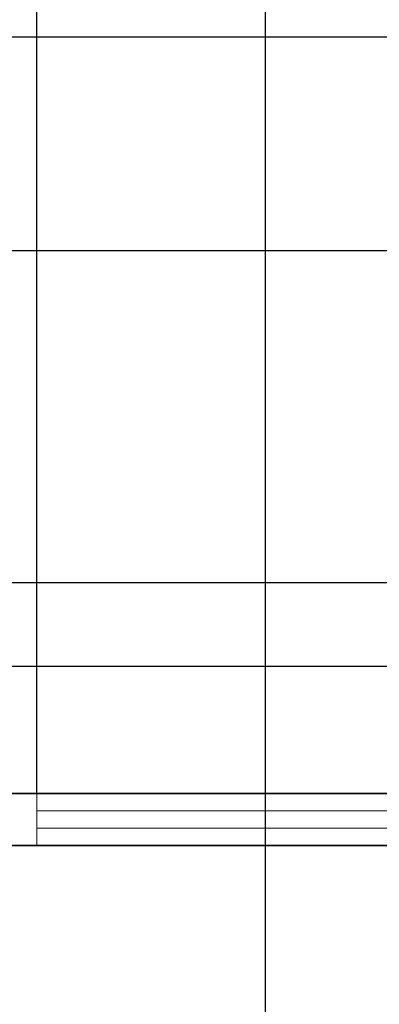
# Model space of a CAD drawing. Units: inches. Extents: x -26 to 385, y 12 to 697.
# Tile 4 of 13: x 192 to 223, y 130 to 215. Entities that reach past the tile are written whole.
import ezdxf

# ---------------------------------------------------------------- set-up
doc = ezdxf.new("R2010")
doc.units = ezdxf.units.IN
doc.header["$MEASUREMENT"] = 0
for name, color, linetype, lineweight in [('A-ANNO-DIMS', 4, 'Continuous', 18), ('A-GLAZ', 5, 'Continuous', 18), ('A-WALL', 40, 'Continuous', 35)]:
    doc.layers.add(name, color=color, linetype=linetype, lineweight=lineweight)
doc.styles.get("Standard").update_dxf_attribs({"font": 'italic8.shx'})
doc.dimstyles.get("Standard").update_dxf_attribs({"dimtxt": 8, "dimasz": 0.18, "dimexe": 0.18, "dimexo": 0.0625, "dimgap": 0.09, "dimtad": 0, "dimtih": 1, "dimtoh": 1, "dimdec": 4, "dimzin": 0, "dimdsep": 46, "dimlunit": 3, "dimtxsty": 'Standard', "dimcen": 0.09, "dimclrd": 2, "dimclre": 3, "dimclrt": 6, "dimadec": 0, "dimazin": 0, "dimtfac": 1, "dimtdec": 4, "dimtofl": 0, "dimtmove": 0, "dimatfit": 3, "dimfxl": 1, "dimtolj": 1, "dimtzin": 0, "dimarcsym": 0})

# ---------------------------------------------------------------- blocks, each defined once
blk = doc.blocks.new('*D28')
at = {"layer": 'A-ANNO-DIMS', "color": 3, "lineweight": -2, "transparency": 16777216}
for p, q in [((141.692, 194.903), (355.559, 194.903)), ((141.692, 158.903), (355.559, 158.903))]:
    blk.add_line(p, q, dxfattribs=at)
at = {"layer": 'A-ANNO-DIMS', "color": 2, "lineweight": -2, "transparency": 16777216}
for p, q in [((355.379, 194.723), (355.379, 181.755)), ((355.379, 159.083), (355.379, 172.052))]:
    blk.add_line(p, q, dxfattribs=at)
at = {"layer": 'A-ANNO-DIMS', "color": 2, "transparency": 16777216}
for points in [[(355.349, 194.723), (355.409, 194.723), (355.379, 194.903)], [(355.349, 159.083), (355.409, 159.083), (355.379, 158.903)]]:
    blk.add_solid(points, dxfattribs=at)
at = {"layer": 'Defpoints', "color": 0, "transparency": 16777216}
for p in [(141.629, 194.903), (355.379, 194.903), (141.629, 158.903)]:
    blk.add_point(p, dxfattribs=at)
at = {"layer": 'A-ANNO-DIMS', "color": 6, "transparency": 16777216, "insert": (355.379, 176.903), "char_height": 8, "attachment_point": 5}
blk.add_mtext('\\A1;3\'-0"', dxfattribs=at)
blk = doc.blocks.new('*D32')
at = {"layer": 'A-ANNO-DIMS', "color": 3, "lineweight": -2, "transparency": 16777216}
for p, q in [((239.825, 213.385), (-5.301, 213.385)), ((239.825, 166.141), (-5.301, 166.141))]:
    blk.add_line(p, q, dxfattribs=at)
at = {"layer": 'A-ANNO-DIMS', "color": 2, "lineweight": -2, "transparency": 16777216}
for p, q in [((-5.121, 213.205), (-5.121, 194.615)), ((-5.121, 166.321), (-5.121, 184.911))]:
    blk.add_line(p, q, dxfattribs=at)
at = {"layer": 'A-ANNO-DIMS', "color": 2, "transparency": 16777216}
for points in [[(-5.151, 213.205), (-5.091, 213.205), (-5.121, 213.385)], [(-5.151, 166.321), (-5.091, 166.321), (-5.121, 166.141)]]:
    blk.add_solid(points, dxfattribs=at)
at = {"layer": 'Defpoints', "color": 0, "transparency": 16777216}
for p in [(-5.121, 213.385), (239.888, 213.385), (239.888, 166.141)]:
    blk.add_point(p, dxfattribs=at)
at = {"layer": 'A-ANNO-DIMS', "color": 6, "transparency": 16777216, "insert": (-5.121, 189.763), "char_height": 8, "attachment_point": 5}
blk.add_mtext('\\A1;3\'-11"', dxfattribs=at)
blk = doc.blocks.new('*D35')
at = {"layer": 'A-ANNO-DIMS', "color": 3, "lineweight": -2, "transparency": 16777216}
for p, q in [((193.598, 147.942), (193.598, 684.809)), ((244.986, 147.942), (244.986, 684.809))]:
    blk.add_line(p, q, dxfattribs=at)
at = {"layer": 'A-ANNO-DIMS', "color": 2, "lineweight": -2, "transparency": 16777216}
for p, q in [((193.778, 684.629), (244.806, 684.629)), ((244.986, 684.629), (245.166, 684.629))]:
    blk.add_line(p, q, dxfattribs=at)
at = {"layer": 'A-ANNO-DIMS', "color": 2, "transparency": 16777216}
for points in [[(193.778, 684.659), (193.778, 684.599), (193.598, 684.629)], [(244.806, 684.659), (244.806, 684.599), (244.986, 684.629)]]:
    blk.add_solid(points, dxfattribs=at)
at = {"layer": 'Defpoints', "color": 0, "transparency": 16777216}
for p in [(244.986, 684.629), (193.598, 147.879), (244.986, 147.879)]:
    blk.add_point(p, dxfattribs=at)
at = {"layer": 'A-ANNO-DIMS', "color": 6, "transparency": 16777216, "insert": (278.398, 684.629), "char_height": 8, "attachment_point": 5}
blk.add_mtext('\\A1;4\'-3 1/2"', dxfattribs=at)
blk = doc.blocks.new('*D36')
at = {"layer": 'A-ANNO-DIMS', "color": 3, "lineweight": -2, "transparency": 16777216}
for p, q in [((146.129, 147.942), (146.129, 684.809)), ((193.598, 147.942), (193.598, 684.809))]:
    blk.add_line(p, q, dxfattribs=at)
at = {"layer": 'A-ANNO-DIMS', "color": 2, "lineweight": -2, "transparency": 16777216}
for p, q in [((146.309, 684.629), (193.418, 684.629)), ((193.598, 684.629), (193.778, 684.629))]:
    blk.add_line(p, q, dxfattribs=at)
at = {"layer": 'A-ANNO-DIMS', "color": 2, "transparency": 16777216}
for points in [[(146.309, 684.659), (146.309, 684.599), (146.129, 684.629)], [(193.418, 684.659), (193.418, 684.599), (193.598, 684.629)]]:
    blk.add_solid(points, dxfattribs=at)
at = {"layer": 'Defpoints', "color": 0, "transparency": 16777216}
for p in [(193.598, 684.629), (146.129, 147.879), (193.598, 147.879)]:
    blk.add_point(p, dxfattribs=at)
at = {"layer": 'A-ANNO-DIMS', "color": 6, "transparency": 16777216, "insert": (228.344, 684.629), "char_height": 8, "attachment_point": 5}
blk.add_mtext('\\A1;3\'-11 1/2"', dxfattribs=at)
blk = doc.blocks.new('*D39')
at = {"layer": 'A-ANNO-DIMS', "color": 3, "lineweight": -2, "transparency": 16777216}
for p, q in [((183.359, 597.317), (183.359, 23.949)), ((213.359, 597.317), (213.359, 23.949))]:
    blk.add_line(p, q, dxfattribs=at)
at = {"layer": 'A-ANNO-DIMS', "color": 2, "lineweight": -2, "transparency": 16777216}
for p, q in [((183.539, 24.129), (213.179, 24.129)), ((213.359, 24.129), (213.539, 24.129))]:
    blk.add_line(p, q, dxfattribs=at)
at = {"layer": 'A-ANNO-DIMS', "color": 2, "transparency": 16777216}
for points in [[(183.539, 24.159), (183.539, 24.099), (183.359, 24.129)], [(213.179, 24.159), (213.179, 24.099), (213.359, 24.129)]]:
    blk.add_solid(points, dxfattribs=at)
at = {"layer": 'Defpoints', "color": 0, "transparency": 16777216}
for p in [(183.359, 597.379), (213.359, 597.379), (213.359, 24.129)]:
    blk.add_point(p, dxfattribs=at)
at = {"layer": 'A-ANNO-DIMS', "color": 6, "transparency": 16777216, "insert": (231.533, 24.129), "char_height": 8, "attachment_point": 5}
blk.add_mtext('\\A1;2\'-6"', dxfattribs=at)
blk = doc.blocks.new('*D55')
at = {"layer": 'A-ANNO-DIMS', "color": 3, "lineweight": -2, "transparency": 16777216}
for p, q in [((146.192, 158.903), (355.559, 158.903)), ((146.192, 147.879), (355.559, 147.879))]:
    blk.add_line(p, q, dxfattribs=at)
at = {"layer": 'A-ANNO-DIMS', "color": 2, "lineweight": -2, "transparency": 16777216}
for p, q in [((355.379, 158.723), (355.379, 158.243)), ((355.379, 148.059), (355.379, 148.539))]:
    blk.add_line(p, q, dxfattribs=at)
at = {"layer": 'A-ANNO-DIMS', "color": 2, "transparency": 16777216}
for points in [[(355.349, 158.723), (355.409, 158.723), (355.379, 158.903)], [(355.349, 148.059), (355.409, 148.059), (355.379, 147.879)]]:
    blk.add_solid(points, dxfattribs=at)
at = {"layer": 'Defpoints', "color": 0, "transparency": 16777216}
for p in [(146.129, 158.903), (355.379, 158.903), (146.129, 147.879)]:
    blk.add_point(p, dxfattribs=at)
at = {"layer": 'A-ANNO-DIMS', "color": 6, "transparency": 16777216, "insert": (355.379, 153.391), "char_height": 8, "attachment_point": 5}
blk.add_mtext('\\A1;0\'-11"', dxfattribs=at)

msp = doc.modelspace()

# ---------------------------------------------------------------- linework, layer by layer
at = {"layer": 'A-GLAZ'}
for p, q in [((193.59818, 147.87909), (193.59818, 143.37909)), ((244.98557, 147.87909), (193.59818, 147.87909)), ((193.59818, 146.37909), (244.98557, 146.37909)), ((193.59818, 144.87909), (244.98557, 144.87909)), ((193.59818, 143.37909), (244.98557, 143.37909))]:
    msp.add_line(p, q, dxfattribs=at)
at = {"layer": 'A-WALL'}
for p, q in [((320.62932, 147.87909), (146.12932, 147.87909)), ((320.62932, 143.37909), (141.62932, 143.37909))]:
    msp.add_line(p, q, dxfattribs=at)

# ---------------------------------------------------------------- dimensions: what is measured, and where the dimension line sits
at = {"layer": 'A-ANNO-DIMS'}
for base, p1, p2, picture, middle in [((193.59818, 684.62909), (146.12932, 147.87909), (193.59818, 147.87909), '*D36', (228.34437, 684.62909)), ((244.98557, 684.62909), (193.59818, 147.87909), (244.98557, 147.87909), '*D35', (278.39843, 684.62909)), ((213.35855, 24.12909), (183.35855, 597.37909), (213.35855, 597.37909), '*D39', (231.53331, 24.12909))]:
    dim = msp.add_linear_dim(base=base, p1=p1, p2=p2, dimstyle='Standard', override={"dimdec": 1, "dimlfac": 1, "dimrnd": 0, "dimzin": 1, "dimdsep": 46, "dimlunit": 4, "dimfrac": 2}, dxfattribs=at)
    dim.commit()
    dim.dimension.update_dxf_attribs({"geometry": picture, "text_midpoint": middle})
for base, p1, p2, picture, middle in [((-5.12068, 213.38513), (239.88756, 166.14113), (239.88756, 213.38513), '*D32', (-5.12068, 189.76313)), ((355.37932, 194.90341), (141.62932, 158.90341), (141.62932, 194.90341), '*D28', (355.37932, 176.90341)), ((355.37932, 158.90341), (146.12932, 147.87909), (146.12932, 158.90341), '*D55', (355.37932, 153.39125))]:
    dim = msp.add_linear_dim(base=base, p1=p1, p2=p2, angle=90, dimstyle='Standard', override={"dimdec": 1, "dimlfac": 1, "dimrnd": 0, "dimzin": 1, "dimdsep": 46, "dimlunit": 4, "dimfrac": 2}, dxfattribs=at)
    dim.commit()
    dim.dimension.update_dxf_attribs({"geometry": picture, "text_midpoint": middle})

doc.saveas('drawing.dxf')
